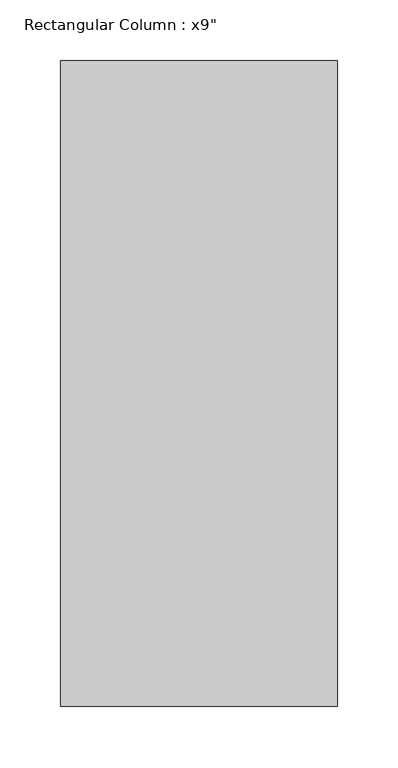
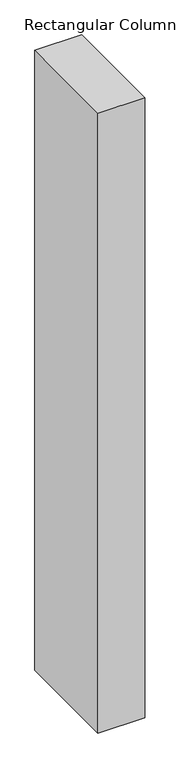
"""IFC4 building model written with IfcOpenShell, lengths in millimetres: column geometry."""

from ifc_helpers import new_model, si_unit, frame, origin, place, context, project, spatial, polyline, outline, extrude, source, transform, mapped, element, save


def column_c97b5c1c(model_context):
    return source(origin(), model_context, "Body", "SweptSolid", [
        extrude(outline(polyline([(114.3, 266.7), (114.3, -266.7), (-114.3, -266.7), (-114.3, 266.7), (114.3, 266.7)])), frame((0.0, 0.0, 9601.2), z_axis=(0.0, 0.0, 1.0), x_axis=(1.0, 0.0, 0.0)), (0.0, 0.0, 1.0), 3200.4),
    ])


if __name__ == "__main__":
    model = new_model("IFC4")
    model_context = context("Model", 3, world=origin())
    ifc_project = project(units=[si_unit("LENGTHUNIT", "METRE", prefix="MILLI")], contexts=[model_context])
    site = spatial("IfcSite", under=ifc_project)
    building = spatial("IfcBuilding", under=site)
    placement = place(None, origin())
    column_shape = column_c97b5c1c(model_context)
    element("IfcColumn", 1, ObjectType="Rectangular Column : x9\"", at=placement, inside=building, context=model_context, shape_type="MappedRepresentation", body=[
        mapped(column_shape, transform((0.0, 0.0, 0.0), x_axis=(1.0, 0.0, 0.0), y_axis=(0.0, 1.0, 0.0), z_axis=(0.0, 0.0, 1.0))),
    ])
    save(model, "model.ifc")

# Revit data of these elements
# Type "Rectangular Column : x9\""
#   Assembly Code = "B1010200"
#   Depth = 1' - 9"
#   Offset Base = 0' - 0"
#   Offset Top = 0' - 0"
#   Width = 0' - 9"
#   Material = none
